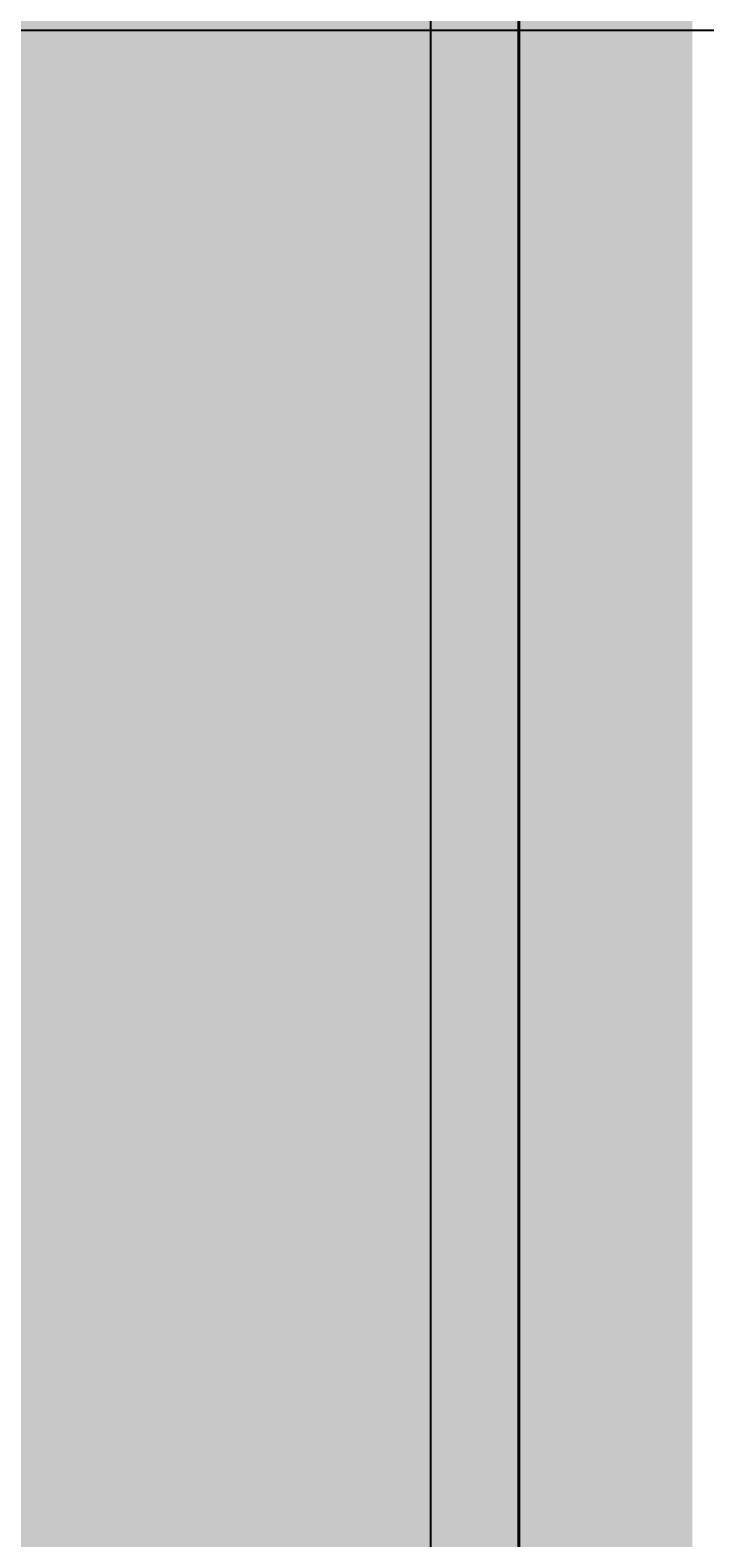
# Model space of a CAD drawing. Units: feet. Extents: x 2695 to 2912, y 795 to 1139.
# Tile 63 of 83: x 2877 to 2896, y 979 to 1021. Entities that reach past the tile are written whole.
import ezdxf

# ---------------------------------------------------------------- set-up
doc = ezdxf.new("R2010")
doc.units = ezdxf.units.FT
for name, color, linetype, lineweight in [('A-ANNO-DIMS', 2, 'Continuous', 18), ('A-ELEV', 7, 'Continuous', 35), ('A-ELEV-PATT', 252, 'Continuous', 13)]:
    doc.layers.add(name, color=color, linetype=linetype, lineweight=lineweight)
doc.styles.get("Standard").update_dxf_attribs({"font": 'arial.ttf'})
doc.dimstyles.get("Standard").update_dxf_attribs({"dimtxt": 0.18, "dimasz": 0.18, "dimexe": 0.18, "dimexo": 0.0625, "dimgap": 0.09, "dimtad": 0, "dimtih": 1, "dimtoh": 1, "dimdec": 1, "dimzin": 0, "dimdsep": 46, "dimlunit": 3, "dimtxsty": 'Standard', "dimcen": 0.09, "dimadec": 0, "dimazin": 0, "dimtfac": 1, "dimtdec": 1, "dimtofl": 0, "dimtmove": 0, "dimatfit": 3, "dimfxl": 1, "dimtolj": 1, "dimtzin": 0, "dimarcsym": 0})

# ---------------------------------------------------------------- blocks, each defined once
blk = doc.blocks.new('*D17')
at = {"layer": 'A-ANNO-DIMS', "color": 0, "lineweight": -2, "transparency": 16777216}
for p, q in [((2843.637, 1020.824), (2911.424, 1020.824)), ((2911.244, 1020.644), (2911.244, 979.059)), ((2911.244, 937.111), (2911.244, 978.695)), ((2890.699, 936.931), (2911.424, 936.931))]:
    blk.add_line(p, q, dxfattribs=at)
at = {"layer": 'A-ANNO-DIMS', "color": 0, "transparency": 16777216}
for points in [[(2911.214, 1020.644), (2911.274, 1020.644), (2911.244, 1020.824)], [(2911.214, 937.111), (2911.274, 937.111), (2911.244, 936.931)]]:
    blk.add_solid(points, dxfattribs=at)
at = {"layer": 'Defpoints', "color": 0, "transparency": 16777216}
for p in [(2843.575, 1020.824), (2911.244, 1020.824), (2890.636, 936.931)]:
    blk.add_point(p, dxfattribs=at)
at = {"layer": 'A-ANNO-DIMS', "color": 0, "transparency": 16777216, "insert": (2911.244, 978.877), "char_height": 0.18, "attachment_point": 5}
blk.add_mtext('\\A1;83.9', dxfattribs=at)
blk = doc.blocks.new('*D50')
at = {"layer": 'A-ANNO-DIMS', "color": 0, "lineweight": -2, "transparency": 16777216}
for p, q in [((2810.041, 972.03), (2810.041, 1138.886)), ((2888.188, 972.03), (2888.188, 1138.886)), ((2810.221, 1138.706), (2848.721, 1138.706)), ((2888.008, 1138.706), (2849.508, 1138.706))]:
    blk.add_line(p, q, dxfattribs=at)
at = {"layer": 'A-ANNO-DIMS', "color": 0, "transparency": 16777216}
for points in [[(2810.221, 1138.736), (2810.221, 1138.676), (2810.041, 1138.706)], [(2888.008, 1138.736), (2888.008, 1138.676), (2888.188, 1138.706)]]:
    blk.add_solid(points, dxfattribs=at)
at = {"layer": 'Defpoints', "color": 0, "transparency": 16777216}
for p in [(2888.188, 1138.706), (2810.041, 971.967), (2888.188, 971.967)]:
    blk.add_point(p, dxfattribs=at)
at = {"layer": 'A-ANNO-DIMS', "color": 0, "transparency": 16777216, "insert": (2849.114, 1138.706), "char_height": 0.18, "attachment_point": 5}
blk.add_mtext('\\A1;78.15', dxfattribs=at)
blk = doc.blocks.new('*D51')
at = {"layer": 'A-ANNO-DIMS', "color": 0, "lineweight": -2, "transparency": 16777216}
for p, q in [((2888.188, 972.03), (2888.188, 1138.886)), ((2890.636, 972.03), (2890.636, 1138.886)), ((2888.368, 1138.706), (2889.017, 1138.706)), ((2890.456, 1138.706), (2889.808, 1138.706))]:
    blk.add_line(p, q, dxfattribs=at)
at = {"layer": 'A-ANNO-DIMS', "color": 0, "transparency": 16777216}
for points in [[(2888.368, 1138.736), (2888.368, 1138.676), (2888.188, 1138.706)], [(2890.456, 1138.736), (2890.456, 1138.676), (2890.636, 1138.706)]]:
    blk.add_solid(points, dxfattribs=at)
at = {"layer": 'Defpoints', "color": 0, "transparency": 16777216}
for p in [(2890.636, 1138.706), (2888.188, 971.967), (2890.636, 971.967)]:
    blk.add_point(p, dxfattribs=at)
at = {"layer": 'A-ANNO-DIMS', "color": 0, "transparency": 16777216, "insert": (2889.412, 1138.706), "char_height": 0.18, "attachment_point": 5}
blk.add_mtext('\\A1;2.448', dxfattribs=at)

msp = doc.modelspace()

# ---------------------------------------------------------------- hatches: boundary and pattern name
at = {"layer": 'A-ELEV-PATT'}
h = msp.add_hatch(color=256, dxfattribs=at)
h.set_gradient(color1=(147, 149, 152), color2=(147, 149, 152), tint=1)
h.paths.add_polyline_path([(2770.6361, 1118.4096), (2710.6361, 1118.4096), (2710.6361, 1062.9306), (2770.6361, 1062.9306)])
h.paths.add_polyline_path([(2890.6361, 1103.3378), (2770.6361, 1103.3378), (2770.6361, 1062.9306), (2890.6361, 1062.9306)])
h.paths.add_polyline_path([(2730.7081, 1048.1052), (2755.1125, 1048.1052), (2755.1125, 936.9306), (2770.6361, 936.9306), (2770.6361, 1050.3105), (2715.8852, 1050.3105), (2715.8852, 936.9306), (2730.7081, 936.9306)])
h.paths.add_polyline_path([(2890.6361, 1050.3105), (2770.6361, 1050.3105), (2770.6361, 971.9673), (2778.0341, 971.9673), (2778.0341, 1020.8235), (2843.575, 1020.8235), (2843.575, 971.9673), (2890.6361, 971.9673)])
h.paths.add_polyline_path([(2888.1882, 970.7156), (2843.575, 970.7156), (2843.575, 964.8267), (2888.1882, 964.8267)])
h.paths.add_polyline_path([(2888.1882, 964.1328), (2843.575, 964.1328), (2843.575, 956.614), (2888.1882, 956.614)])
h.paths.add_polyline_path([(2888.1882, 955.9202), (2843.575, 955.9202), (2843.575, 949.2892), (2888.1882, 949.2892)])
h.paths.add_polyline_path([(2888.1882, 948.5954), (2843.575, 948.5954), (2843.575, 941.3507), (2888.1882, 941.3507)])
h.paths.add_polyline_path([(2888.1882, 940.6569), (2843.575, 940.6569), (2843.575, 936.9306), (2888.1882, 936.9306)])
h.paths.add_polyline_path([(2890.6361, 970.7156), (2888.9368, 970.7156), (2888.9368, 964.8267), (2890.6361, 964.8267)])
h.paths.add_polyline_path([(2890.6361, 964.1328), (2888.9368, 964.1328), (2888.9368, 956.614), (2890.6361, 956.614)])
h.paths.add_polyline_path([(2890.6361, 955.9202), (2888.9368, 955.9202), (2888.9368, 949.2892), (2890.6361, 949.2892)])
h.paths.add_polyline_path([(2890.6361, 940.6569), (2888.9368, 940.6569), (2888.9368, 936.9306), (2890.6361, 936.9306)])
h.paths.add_polyline_path([(2890.6361, 948.5954), (2888.9368, 948.5954), (2888.9368, 941.3507), (2890.6361, 941.3507)])
h.paths.add_polyline_path([(2772.5216, 970.7156), (2770.6361, 970.7156), (2770.6361, 964.8267), (2772.5216, 964.8267)])
h.paths.add_polyline_path([(2772.5216, 964.1328), (2770.6361, 964.1328), (2770.6361, 956.614), (2772.5216, 956.614)])
h.paths.add_polyline_path([(2772.5216, 955.9202), (2770.6361, 955.9202), (2770.6361, 949.2892), (2772.5216, 949.2892)])
h.paths.add_polyline_path([(2772.5216, 948.5954), (2770.6361, 948.5954), (2770.6361, 941.3507), (2772.5216, 941.3507)])
h.paths.add_polyline_path([(2772.5216, 940.6569), (2770.6361, 940.6569), (2770.6361, 936.9306), (2772.5216, 936.9306)])
h.paths.add_polyline_path([(2778.0341, 940.6569), (2773.2702, 940.6569), (2773.2702, 936.9306), (2778.0341, 936.9306)])
h.paths.add_polyline_path([(2778.0341, 970.7156), (2773.2702, 970.7156), (2773.2702, 964.8267), (2778.0341, 964.8267)])
h.paths.add_polyline_path([(2778.0341, 964.1328), (2773.2702, 964.1328), (2773.2702, 956.614), (2778.0341, 956.614)])
h.paths.add_polyline_path([(2778.0341, 955.9202), (2773.2702, 955.9202), (2773.2702, 949.2892), (2778.0341, 949.2892)])
h.paths.add_polyline_path([(2778.0341, 948.5954), (2773.2702, 948.5954), (2773.2702, 941.3507), (2778.0341, 941.3507)])
h.paths.add_polyline_path([(2810.0407, 940.6569), (2780.0341, 940.6569), (2780.0341, 936.9306), (2810.0407, 936.9306)])
h.paths.add_polyline_path([(2890.6361, 924.3105), (2770.6361, 924.3105), (2770.6361, 810.9306), (2773.5029, 810.9306), (2773.5029, 905.5143), (2805.9398, 905.5143), (2838.3767, 905.5143), (2838.3767, 810.9306), (2890.6361, 810.9306)])
h = msp.add_hatch(color=256, dxfattribs=at)
h.set_gradient(color1=(255, 255, 255), tint=1)
h.paths.add_polyline_path([(2895.4694, 1107.8588), (2890.6361, 1107.8588), (2890.6361, 810.9306), (2895.4694, 810.9306)])
h = msp.add_hatch(color=256, dxfattribs=at)
h.set_gradient(color1=(255, 255, 255), tint=1)
h.paths.add_polyline_path([(2890.6361, 1050.3105), (2881.9484, 1050.3105), (2881.9484, 971.9673), (2890.6361, 971.9673)])
h.paths.add_polyline_path([(2888.1882, 970.7156), (2881.9484, 970.7156), (2881.9484, 964.8267), (2888.1882, 964.8267)])
h.paths.add_polyline_path([(2890.6361, 970.7156), (2888.9368, 970.7156), (2888.9368, 964.8267), (2890.6361, 964.8267)])
h.paths.add_polyline_path([(2888.1882, 964.1328), (2881.9484, 964.1328), (2881.9484, 956.614), (2888.1882, 956.614)])
h.paths.add_polyline_path([(2890.6361, 964.1328), (2888.9368, 964.1328), (2888.9368, 956.614), (2890.6361, 956.614)])
h.paths.add_polyline_path([(2888.1882, 955.9202), (2881.9484, 955.9202), (2881.9484, 949.2892), (2888.1882, 949.2892)])
h.paths.add_polyline_path([(2890.6361, 955.9202), (2888.9368, 955.9202), (2888.9368, 949.2892), (2890.6361, 949.2892)])
h.paths.add_polyline_path([(2888.1882, 948.5954), (2881.9484, 948.5954), (2881.9484, 941.3507), (2888.1882, 941.3507)])
h.paths.add_polyline_path([(2890.6361, 948.5954), (2888.9368, 948.5954), (2888.9368, 941.3507), (2890.6361, 941.3507)])
h.paths.add_polyline_path([(2888.1882, 940.6569), (2881.9484, 940.6569), (2881.9484, 936.9306), (2888.1882, 936.9306)])

# ---------------------------------------------------------------- linework, layer by layer
at = {"layer": 'A-ELEV'}
for p, q in [((2890.6361, 810.9306), (2890.6361, 1107.8588)), ((2890.6361, 1062.9306), (2890.6361, 810.9306))]:
    msp.add_line(p, q, dxfattribs=at)

# ---------------------------------------------------------------- dimensions: what is measured, and where the dimension line sits
at = {"layer": 'A-ANNO-DIMS'}
for base, p1, p2, override, picture, middle in [((2888.1882, 1138.7056), (2810.0407, 971.9673), (2888.1882, 971.9673), {"dimdec": 2, "dimlfac": 1, "dimrnd": 0, "dimzin": 0, "dimdsep": 46, "dimlunit": 2}, '*D50', (2849.1144, 1138.7056)), ((2890.6361, 1138.7056), (2888.1882, 971.9673), (2890.6361, 971.9673), {"dimdec": 3, "dimlfac": 1, "dimrnd": 0, "dimzin": 0, "dimdsep": 46, "dimlunit": 2}, '*D51', (2889.4121, 1138.7056))]:
    dim = msp.add_linear_dim(base=base, p1=p1, p2=p2, dimstyle='Standard', override=override, dxfattribs=at)
    dim.commit()
    dim.dimension.update_dxf_attribs({"geometry": picture, "text_midpoint": middle})
dim = msp.add_linear_dim(base=(2911.2444, 1020.8235), p1=(2890.6361, 936.9306), p2=(2843.575, 1020.8235), angle=90, dimstyle='Standard', override={"dimdec": 1, "dimlfac": 1, "dimrnd": 0, "dimzin": 0, "dimdsep": 46, "dimlunit": 2}, dxfattribs=at)
dim.commit()
dim.dimension.update_dxf_attribs({"geometry": '*D17', "text_midpoint": (2911.2444, 978.877)})

doc.saveas('drawing.dxf')
